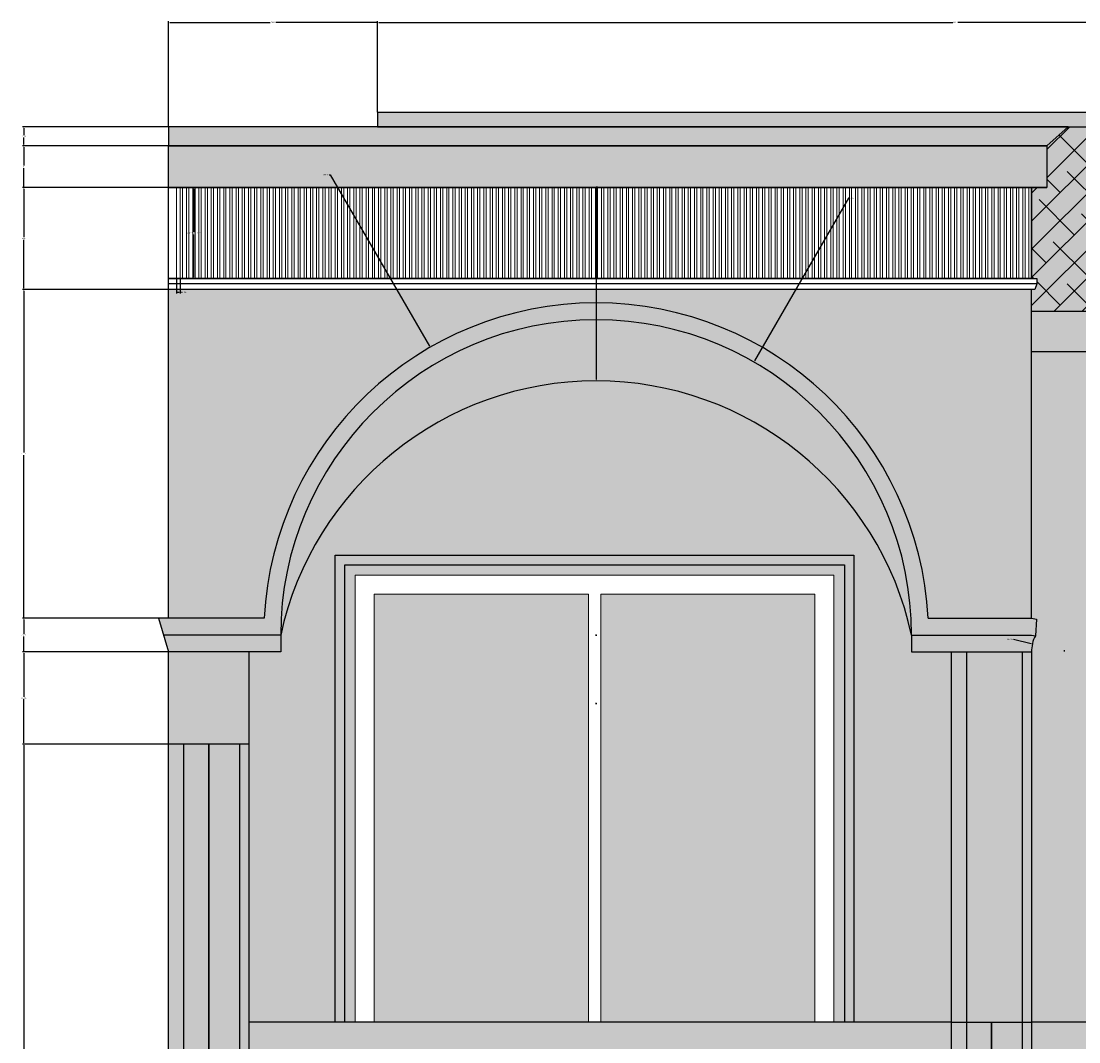
# Model space of a CAD drawing. Units: feet. Extents: x 2352 to 2983, y 950 to 1233.
# Tile 2 of 5: x 2352 to 2504, y 1086 to 1233. Entities that reach past the tile are written whole.
import ezdxf

# ---------------------------------------------------------------- set-up
doc = ezdxf.new("R2010")
doc.units = ezdxf.units.FT
for name, color, linetype, lineweight in [('A-ANNO-DIMS', 2, 'Continuous', 18), ('A-ELEV', 7, 'Continuous', 25), ('A-ELEV-DETL', 8, 'Continuous', 13), ('A-ELEV-PATT', 252, 'Continuous', 13), ('A-GLAZ', 4, 'Continuous', 18)]:
    doc.layers.add(name, color=color, linetype=linetype, lineweight=lineweight)
doc.styles.get("Standard").update_dxf_attribs({"font": 'arial.ttf'})
doc.dimstyles.get("Standard").update_dxf_attribs({"dimtxt": 0.18, "dimasz": 0.18, "dimexe": 0.18, "dimexo": 0.0625, "dimgap": 0.09, "dimtad": 0, "dimtih": 1, "dimtoh": 1, "dimdec": 1, "dimzin": 0, "dimdsep": 46, "dimlunit": 3, "dimtxsty": 'Standard', "dimcen": 0.09, "dimadec": 0, "dimazin": 0, "dimtfac": 1, "dimtdec": 1, "dimtofl": 0, "dimtmove": 0, "dimatfit": 3, "dimfxl": 1, "dimtolj": 1, "dimtzin": 0, "dimarcsym": 0})

# ---------------------------------------------------------------- blocks, each defined once
blk = doc.blocks.new('GRILLE-SLAT')
blk.add_lwpolyline([(0, 13.08), (0.56, 13.08), (0.56, 0), (0, 0)], close=True)
blk.add_lwpolyline([(0, 13.08), (0.56, 13.08), (0.56, 0), (0, 0)], close=True)
blk = doc.blocks.new('*D5')
at = {"layer": 'A-ANNO-DIMS', "color": 0, "lineweight": -2, "transparency": 16777216}
for p, q in [((2375.04, 1209.01), (2377.12, 1209.01)), ((2376.94, 1208.83), (2376.94, 1202.66)), ((2376.94, 1196.12), (2376.94, 1202.29)), ((2375.04, 1195.94), (2377.12, 1195.94))]:
    blk.add_line(p, q, dxfattribs=at)
at = {"layer": 'A-ANNO-DIMS', "color": 0, "transparency": 16777216}
for points in [[(2376.91, 1208.83), (2376.97, 1208.83), (2376.94, 1209.01)], [(2376.91, 1196.12), (2376.97, 1196.12), (2376.94, 1195.94)]]:
    blk.add_solid(points, dxfattribs=at)
at = {"layer": 'Defpoints', "color": 0, "transparency": 16777216}
for p in [(2374.98, 1209.01), (2376.94, 1209.01), (2374.98, 1195.94)]:
    blk.add_point(p, dxfattribs=at)
at = {"layer": 'A-ANNO-DIMS', "color": 0, "transparency": 16777216, "insert": (2376.94, 1202.47), "char_height": 0.18, "attachment_point": 5}
blk.add_mtext('\\A1;GRILLE SLAT 13 TYP.', dxfattribs=at)
blk = doc.blocks.new('*D6')
at = {"layer": 'A-ANNO-DIMS', "color": 0, "lineweight": -2, "transparency": 16777216}
for p, q in [((2374.42, 1195.87), (2374.42, 1193.79)), ((2374.98, 1195.87), (2374.98, 1193.79)), ((2374.6, 1193.97), (2374.8, 1193.97)), ((2374.98, 1193.97), (2375.16, 1193.97))]:
    blk.add_line(p, q, dxfattribs=at)
at = {"layer": 'A-ANNO-DIMS', "color": 0, "transparency": 16777216}
for points in [[(2374.6, 1194), (2374.6, 1193.94), (2374.42, 1193.97)], [(2374.8, 1194), (2374.8, 1193.94), (2374.98, 1193.97)]]:
    blk.add_solid(points, dxfattribs=at)
at = {"layer": 'Defpoints', "color": 0, "transparency": 16777216}
for p in [(2374.42, 1195.94), (2374.98, 1195.94), (2374.98, 1193.97)]:
    blk.add_point(p, dxfattribs=at)
at = {"layer": 'A-ANNO-DIMS', "color": 0, "transparency": 16777216, "insert": (2375.61, 1193.97), "char_height": 0.18, "attachment_point": 5}
blk.add_mtext('\\A1;1 TYP.', dxfattribs=at)
blk = doc.blocks.new('*D8')
at = {"layer": 'A-ANNO-DIMS', "color": 0, "lineweight": -2, "transparency": 16777216}
for p, q in [((2373.3, 1217.81), (2373.3, 1232.95)), ((2403.34, 1219.88), (2403.34, 1232.95)), ((2373.48, 1232.77), (2387.92, 1232.77)), ((2403.16, 1232.77), (2388.71, 1232.77))]:
    blk.add_line(p, q, dxfattribs=at)
at = {"layer": 'A-ANNO-DIMS', "color": 0, "transparency": 16777216}
for points in [[(2373.48, 1232.8), (2373.48, 1232.74), (2373.3, 1232.77)], [(2403.16, 1232.8), (2403.16, 1232.74), (2403.34, 1232.77)]]:
    blk.add_solid(points, dxfattribs=at)
at = {"layer": 'Defpoints', "color": 0, "transparency": 16777216}
for p in [(2403.34, 1232.77), (2403.34, 1219.82), (2373.3, 1217.75)]:
    blk.add_point(p, dxfattribs=at)
at = {"layer": 'A-ANNO-DIMS', "color": 0, "transparency": 16777216, "insert": (2388.32, 1232.77), "char_height": 0.18, "attachment_point": 5}
blk.add_mtext('\\A1;30.04', dxfattribs=at)
blk = doc.blocks.new('*D9')
at = {"layer": 'A-ANNO-DIMS', "color": 0, "lineweight": -2, "transparency": 16777216}
for p, q in [((2403.34, 1219.88), (2403.34, 1232.95)), ((2569.44, 1219.88), (2569.44, 1232.95)), ((2403.52, 1232.77), (2486.02, 1232.77)), ((2569.26, 1232.77), (2486.76, 1232.77))]:
    blk.add_line(p, q, dxfattribs=at)
at = {"layer": 'A-ANNO-DIMS', "color": 0, "transparency": 16777216}
for points in [[(2403.52, 1232.8), (2403.52, 1232.74), (2403.34, 1232.77)], [(2569.26, 1232.8), (2569.26, 1232.74), (2569.44, 1232.77)]]:
    blk.add_solid(points, dxfattribs=at)
at = {"layer": 'Defpoints', "color": 0, "transparency": 16777216}
for p in [(2569.44, 1232.77), (2403.34, 1219.82), (2569.44, 1219.82)]:
    blk.add_point(p, dxfattribs=at)
at = {"layer": 'A-ANNO-DIMS', "color": 0, "transparency": 16777216, "insert": (2486.39, 1232.77), "char_height": 0.18, "attachment_point": 5}
blk.add_mtext('\\A1;166.1', dxfattribs=at)
blk = doc.blocks.new('*D23')
at = {"layer": 'A-ANNO-DIMS', "color": 0, "lineweight": -2, "transparency": 16777216}
for p, q in [((2373.23, 1129.01), (2352.3, 1129.01)), ((2352.48, 1128.83), (2352.48, 1077.3)), ((2352.48, 1025.39), (2352.48, 1076.93)), ((2365.37, 1025.21), (2352.3, 1025.21))]:
    blk.add_line(p, q, dxfattribs=at)
at = {"layer": 'A-ANNO-DIMS', "color": 0, "transparency": 16777216}
for points in [[(2352.45, 1128.83), (2352.51, 1128.83), (2352.48, 1129.01)], [(2352.45, 1025.39), (2352.51, 1025.39), (2352.48, 1025.21)]]:
    blk.add_solid(points, dxfattribs=at)
at = {"layer": 'Defpoints', "color": 0, "transparency": 16777216}
for p in [(2352.48, 1129.01), (2373.3, 1129.01), (2365.43, 1025.21)]:
    blk.add_point(p, dxfattribs=at)
at = {"layer": 'A-ANNO-DIMS', "color": 0, "transparency": 16777216, "insert": (2352.48, 1077.11), "char_height": 0.18, "attachment_point": 5}
blk.add_mtext('\\A1;103.8', dxfattribs=at)
blk = doc.blocks.new('*D24')
at = {"layer": 'A-ANNO-DIMS', "color": 0, "lineweight": -2, "transparency": 16777216}
for p, q in [((2373.23, 1142.24), (2352.3, 1142.24)), ((2352.48, 1142.06), (2352.48, 1135.81)), ((2352.48, 1129.19), (2352.48, 1135.44)), ((2373.23, 1129.01), (2352.3, 1129.01))]:
    blk.add_line(p, q, dxfattribs=at)
at = {"layer": 'A-ANNO-DIMS', "color": 0, "transparency": 16777216}
for points in [[(2352.45, 1142.06), (2352.51, 1142.06), (2352.48, 1142.24)], [(2352.45, 1129.19), (2352.51, 1129.19), (2352.48, 1129.01)]]:
    blk.add_solid(points, dxfattribs=at)
at = {"layer": 'Defpoints', "color": 0, "transparency": 16777216}
for p in [(2352.48, 1142.24), (2373.3, 1142.24), (2373.3, 1129.01)]:
    blk.add_point(p, dxfattribs=at)
at = {"layer": 'A-ANNO-DIMS', "color": 0, "transparency": 16777216, "insert": (2352.48, 1135.63), "char_height": 0.18, "attachment_point": 5}
blk.add_mtext('\\A1;13.224', dxfattribs=at)
blk = doc.blocks.new('*D25')
at = {"layer": 'A-ANNO-DIMS', "color": 0, "lineweight": -2, "transparency": 16777216}
for p, q in [((2371.8, 1147.09), (2352.3, 1147.09)), ((2352.48, 1146.91), (2352.48, 1144.85)), ((2352.48, 1142.42), (2352.48, 1144.48)), ((2373.23, 1142.24), (2352.3, 1142.24))]:
    blk.add_line(p, q, dxfattribs=at)
at = {"layer": 'A-ANNO-DIMS', "color": 0, "transparency": 16777216}
for points in [[(2352.45, 1146.91), (2352.51, 1146.91), (2352.48, 1147.09)], [(2352.45, 1142.42), (2352.51, 1142.42), (2352.48, 1142.24)]]:
    blk.add_solid(points, dxfattribs=at)
at = {"layer": 'Defpoints', "color": 0, "transparency": 16777216}
for p in [(2352.48, 1147.09), (2371.86, 1147.09), (2373.3, 1142.24)]:
    blk.add_point(p, dxfattribs=at)
at = {"layer": 'A-ANNO-DIMS', "color": 0, "transparency": 16777216, "insert": (2352.48, 1144.67), "char_height": 0.18, "attachment_point": 5}
blk.add_mtext('\\A1;4.853', dxfattribs=at)
blk = doc.blocks.new('*D26')
at = {"layer": 'A-ANNO-DIMS', "color": 0, "lineweight": -2, "transparency": 16777216}
for p, q in [((2373.23, 1194.37), (2352.3, 1194.37)), ((2352.48, 1194.19), (2352.48, 1170.91)), ((2352.48, 1147.27), (2352.48, 1170.55)), ((2371.8, 1147.09), (2352.3, 1147.09))]:
    blk.add_line(p, q, dxfattribs=at)
at = {"layer": 'A-ANNO-DIMS', "color": 0, "transparency": 16777216}
for points in [[(2352.45, 1194.19), (2352.51, 1194.19), (2352.48, 1194.37)], [(2352.45, 1147.27), (2352.51, 1147.27), (2352.48, 1147.09)]]:
    blk.add_solid(points, dxfattribs=at)
at = {"layer": 'Defpoints', "color": 0, "transparency": 16777216}
for p in [(2352.48, 1194.37), (2373.3, 1194.37), (2371.86, 1147.09)]:
    blk.add_point(p, dxfattribs=at)
at = {"layer": 'A-ANNO-DIMS', "color": 0, "transparency": 16777216, "insert": (2352.48, 1170.73), "char_height": 0.18, "attachment_point": 5}
blk.add_mtext('\\A1;47.28', dxfattribs=at)
blk = doc.blocks.new('*D27')
at = {"layer": 'A-ANNO-DIMS', "color": 0, "lineweight": -2, "transparency": 16777216}
for p, q in [((2373.23, 1209.01), (2352.3, 1209.01)), ((2352.48, 1208.83), (2352.48, 1201.87)), ((2352.48, 1194.55), (2352.48, 1201.51)), ((2373.23, 1194.37), (2352.3, 1194.37))]:
    blk.add_line(p, q, dxfattribs=at)
at = {"layer": 'A-ANNO-DIMS', "color": 0, "transparency": 16777216}
for points in [[(2352.45, 1208.83), (2352.51, 1208.83), (2352.48, 1209.01)], [(2352.45, 1194.55), (2352.51, 1194.55), (2352.48, 1194.37)]]:
    blk.add_solid(points, dxfattribs=at)
at = {"layer": 'Defpoints', "color": 0, "transparency": 16777216}
for p in [(2352.48, 1209.01), (2373.3, 1209.01), (2373.3, 1194.37)]:
    blk.add_point(p, dxfattribs=at)
at = {"layer": 'A-ANNO-DIMS', "color": 0, "transparency": 16777216, "insert": (2352.48, 1201.69), "char_height": 0.18, "attachment_point": 5}
blk.add_mtext('\\A1;14.64', dxfattribs=at)
blk = doc.blocks.new('*D28')
at = {"layer": 'A-ANNO-DIMS', "color": 0, "lineweight": -2, "transparency": 16777216}
for p, q in [((2373.23, 1215.01), (2352.3, 1215.01)), ((2352.48, 1214.83), (2352.48, 1212.19)), ((2352.48, 1209.19), (2352.48, 1211.83)), ((2373.23, 1209.01), (2352.3, 1209.01))]:
    blk.add_line(p, q, dxfattribs=at)
at = {"layer": 'A-ANNO-DIMS', "color": 0, "transparency": 16777216}
for points in [[(2352.45, 1214.83), (2352.51, 1214.83), (2352.48, 1215.01)], [(2352.45, 1209.19), (2352.51, 1209.19), (2352.48, 1209.01)]]:
    blk.add_solid(points, dxfattribs=at)
at = {"layer": 'Defpoints', "color": 0, "transparency": 16777216}
for p in [(2352.48, 1215.01), (2373.3, 1215.01), (2373.3, 1209.01)]:
    blk.add_point(p, dxfattribs=at)
at = {"layer": 'A-ANNO-DIMS', "color": 0, "transparency": 16777216, "insert": (2352.48, 1212.01), "char_height": 0.18, "attachment_point": 5}
blk.add_mtext('\\A1;6', dxfattribs=at)
blk = doc.blocks.new('*D29')
at = {"layer": 'A-ANNO-DIMS', "color": 0, "lineweight": -2, "transparency": 16777216}
for p, q in [((2373.23, 1217.75), (2352.3, 1217.75)), ((2352.48, 1217.57), (2352.48, 1216.56)), ((2352.48, 1215.19), (2352.48, 1216.2)), ((2373.23, 1215.01), (2352.3, 1215.01))]:
    blk.add_line(p, q, dxfattribs=at)
at = {"layer": 'A-ANNO-DIMS', "color": 0, "transparency": 16777216}
for points in [[(2352.45, 1217.57), (2352.51, 1217.57), (2352.48, 1217.75)], [(2352.45, 1215.19), (2352.51, 1215.19), (2352.48, 1215.01)]]:
    blk.add_solid(points, dxfattribs=at)
at = {"layer": 'Defpoints', "color": 0, "transparency": 16777216}
for p in [(2352.48, 1217.75), (2373.3, 1217.75), (2373.3, 1215.01)]:
    blk.add_point(p, dxfattribs=at)
at = {"layer": 'A-ANNO-DIMS', "color": 0, "transparency": 16777216, "insert": (2352.48, 1216.38), "char_height": 0.18, "attachment_point": 5}
blk.add_mtext('\\A1;2.74', dxfattribs=at)
blk = doc.blocks.new('*D60')
at = {"layer": 'A-ANNO-DIMS', "color": 0, "lineweight": -2, "transparency": 16777216}
for p, q in [((2396.36, 1210.86), (2396.54, 1210.86)), ((2396.54, 1210.86), (2410.78, 1186.19)), ((2434.75, 1144.58), (2434.75, 1144.76)), ((2434.66, 1144.67), (2434.84, 1144.67))]:
    blk.add_line(p, q, dxfattribs=at)
at = {"layer": 'A-ANNO-DIMS', "color": 0, "transparency": 16777216}
blk.add_solid([(2410.8, 1186.21), (2410.75, 1186.18), (2410.87, 1186.03)], dxfattribs=at)
at = {"layer": 'Defpoints', "color": 0, "transparency": 16777216}
for p in [(2410.87, 1186.03), (2434.75, 1144.67)]:
    blk.add_point(p, dxfattribs=at)
at = {"layer": 'A-ANNO-DIMS', "color": 0, "transparency": 16777216, "insert": (2395.88, 1210.86), "char_height": 0.18, "attachment_point": 5}
blk.add_mtext('\\A1;R47.77', dxfattribs=at)
blk = doc.blocks.new('*D61')
at = {"layer": 'A-ANNO-DIMS', "color": 0, "lineweight": -2, "transparency": 16777216}
for p, q in [((2434.93, 1209.06), (2434.75, 1209.06)), ((2434.75, 1209.06), (2434.75, 1181.4)), ((2434.66, 1134.83), (2434.84, 1134.83)), ((2434.75, 1134.74), (2434.75, 1134.92))]:
    blk.add_line(p, q, dxfattribs=at)
at = {"layer": 'A-ANNO-DIMS', "color": 0, "transparency": 16777216}
blk.add_solid([(2434.72, 1181.4), (2434.78, 1181.4), (2434.75, 1181.22)], dxfattribs=at)
at = {"layer": 'Defpoints', "color": 0, "transparency": 16777216}
for p in [(2434.75, 1181.22), (2434.75, 1134.83)]:
    blk.add_point(p, dxfattribs=at)
at = {"layer": 'A-ANNO-DIMS', "color": 0, "transparency": 16777216, "insert": (2435.34, 1209.06), "char_height": 0.18, "attachment_point": 5}
blk.add_mtext('\\A1;R46.4', dxfattribs=at)
blk = doc.blocks.new('*D62')
at = {"layer": 'A-ANNO-DIMS', "color": 0, "lineweight": -2, "transparency": 16777216}
for p, q in [((2471.02, 1207.49), (2457.51, 1184.09)), ((2471.2, 1207.49), (2471.02, 1207.49)), ((2434.75, 1144.58), (2434.75, 1144.76)), ((2434.66, 1144.67), (2434.84, 1144.67))]:
    blk.add_line(p, q, dxfattribs=at)
at = {"layer": 'A-ANNO-DIMS', "color": 0, "transparency": 16777216}
blk.add_solid([(2457.48, 1184.1), (2457.54, 1184.07), (2457.42, 1183.93)], dxfattribs=at)
at = {"layer": 'Defpoints', "color": 0, "transparency": 16777216}
for p in [(2457.42, 1183.93), (2434.75, 1144.67)]:
    blk.add_point(p, dxfattribs=at)
at = {"layer": 'A-ANNO-DIMS', "color": 0, "transparency": 16777216, "insert": (2471.68, 1207.49), "char_height": 0.18, "attachment_point": 5}
blk.add_mtext('\\A1;R45.34', dxfattribs=at)
blk = doc.blocks.new('*D65')
at = {"layer": 'A-ANNO-DIMS', "color": 0, "lineweight": -2, "transparency": 16777216}
for p, q in [((2494.71, 1144.07), (2497.28, 1143.48)), ((2501.95, 1142.41), (2502.13, 1142.41)), ((2502.04, 1142.32), (2502.04, 1142.5))]:
    blk.add_line(p, q, dxfattribs=at)
at = {"layer": 'A-ANNO-DIMS', "color": 0, "transparency": 16777216}
blk.add_solid([(2497.29, 1143.51), (2497.27, 1143.45), (2497.46, 1143.44)], dxfattribs=at)
at = {"layer": 'Defpoints', "color": 0, "transparency": 16777216}
for p in [(2497.46, 1143.44), (2502.04, 1142.41)]:
    blk.add_point(p, dxfattribs=at)
at = {"layer": 'A-ANNO-DIMS', "color": 0, "transparency": 16777216, "insert": (2494.23, 1144.07), "char_height": 0.18, "attachment_point": 5}
blk.add_mtext('\\A1;R4.699', dxfattribs=at)

msp = doc.modelspace()

# ---------------------------------------------------------------- hatches: boundary and pattern name
at = {"layer": 'A-ELEV-PATT'}
h = msp.add_hatch(color=256, dxfattribs=at)
h.dxf.hatch_style = 1
h.paths.add_polyline_path([(2499.5465, 1215.0126), (2373.2965, 1215.0126), (2373.2965, 1209.0126), (2499.5465, 1209.0126)])
h.paths.add_polyline_path([(2502.6085, 1217.7513), (2403.3368, 1217.7513), (2373.2965, 1217.7513), (2373.2965, 1215.0126), (2499.5465, 1215.0126)])
h.paths.add_polyline_path([(2569.4416, 1219.8182), (2403.3368, 1219.8182), (2403.3368, 1217.7513), (2569.4416, 1217.7513)])
h.paths.add_polyline_path([(2593.9663, 1076.1207), (2582.4111, 1069.3398), (2582.4111, 1011.4831), (2595.2079, 1011.4831), (2595.2079, 1023.0126), (2594.1881, 1024.8551), (2594.1881, 1026.3357), (2594.1891, 1026.3338, 0.10932946), (2593.9663, 1027.4578)])
h.paths.add_polyline_path([(2602.5286, 1209.0126), (2593.9663, 1209.0126), (2593.9663, 1027.4578), (2595.2079, 1025.2146), (2602.5286, 1025.2146)])
h.paths.add_polyline_path([(2593.9663, 1083.0126), (2497.3422, 1083.0126), (2497.3422, 1076.1207), (2593.9663, 1076.1207)])
h.paths.add_polyline_path([(2485.8114, 1075.3288), (2384.8273, 1075.3288), (2384.8273, 1011.4831), (2398.2572, 1011.4831), (2398.2572, 1042.4514), (2479.5304, 1042.4514), (2479.5304, 1025.2146), (2485.8114, 1025.2146)])
h.paths.add_polyline_path([(2485.8114, 1083.0126), (2383.4779, 1083.0126), (2383.4779, 1076.1207), (2485.8114, 1076.1207)])
h.paths.add_polyline_path([(2495.9928, 1089.0126), (2491.6239, 1089.0126), (2491.6239, 1025.2146), (2495.9928, 1025.2146)])
h.paths.add_polyline_path([(2491.5297, 1089.0126), (2488.0105, 1089.0126), (2488.0105, 1025.2146), (2491.5297, 1025.2146)])
h.paths.add_polyline_path([(2379.0148, 1129.0147), (2375.4956, 1129.0147), (2375.4956, 1025.2146), (2379.0148, 1025.2146)])
h.paths.add_polyline_path([(2383.4779, 1129.0147), (2379.109, 1129.0147), (2379.109, 1025.2146), (2381.1604, 1025.2146), (2383.4779, 1025.8769)])
h.paths.add_polyline_path([(2389.4076, 1144.6653), (2389.4076, 1142.2389), (2384.8273, 1142.2389), (2384.8273, 1089.0126), (2397.2412, 1089.0126), (2397.2412, 1156.1636), (2471.8066, 1156.1636), (2471.8066, 1089.0126), (2485.8114, 1089.0126), (2485.8114, 1142.2389), (2480.0884, 1142.2389), (2480.0884, 1144.6653, 0.80625477)])
h.paths.add_polyline_path([(2389.4076, 1144.6653, -0.80625477), (2480.0884, 1144.6653, 1)])
h.paths.add_polyline_path([(2579.9743, 1185.4477), (2497.3422, 1185.4477), (2497.3422, 1147.0918), (2498.0576, 1146.9764), (2497.8725, 1144.5798, 0.11184527), (2497.3422, 1142.5724), (2497.3422, 1089.0126), (2505.6415, 1089.0126), (2505.6415, 1159.528, -1), (2532.4859, 1159.528), (2532.4859, 1089.0126), (2541.7346, 1089.0126), (2541.7346, 1159.528, -1), (2568.579, 1159.528), (2568.579, 1089.0126), (2579.9743, 1089.0126)])
h.paths.add_polyline_path([(2579.9743, 1191.2362), (2497.3422, 1191.2362), (2497.3422, 1185.4477), (2579.9743, 1185.4477)])
h.paths.add_polyline_path([(2381.1604, 1023.0126), (2367.0741, 1023.0126), (2367.0741, 963.0126), (2381.1604, 963.0126)])
h.paths.add_polyline_path([(2495.2282, 1011.4831), (2495.2282, 1023.0126), (2439.9479, 1023.0126), (2439.9479, 963.0126), (2446.428, 963.0126), (2446.428, 989.9926, -1), (2485.4222, 989.9926), (2485.4222, 963.0126), (2495.2282, 963.0126)])
h.paths.add_polyline_path([(2446.428, 989.9926), (2446.428, 963.0126), (2485.4222, 963.0126), (2485.4222, 989.9926, 1)], flags=17)
h.paths.add_polyline_path([(2603.7702, 1023.0126), (2595.2079, 1023.0126), (2595.2079, 1011.4831), (2595.2079, 963.0126), (2603.7702, 963.0126)])
h.paths.add_polyline_path([(2482.4531, 1147.0918), (2497.3422, 1147.0918), (2497.3422, 1185.4477), (2497.3422, 1194.3715), (2373.2965, 1194.3715), (2373.2965, 1147.0918), (2387.0428, 1147.0918, -0.95042953)])
h.paths.add_polyline_path([(2384.8273, 1142.2389), (2373.2965, 1142.2389), (2373.2965, 1129.0147), (2384.8273, 1129.0147)])
h.paths.add_polyline_path([(2495.9928, 1142.2389), (2488.0105, 1142.2389), (2488.0105, 1089.0126), (2491.5297, 1089.0126), (2495.9928, 1089.0126)])
h = msp.add_hatch(color=256, dxfattribs=at)
h.dxf.hatch_style = 1
h.paths.add_polyline_path([(2595.2079, 1011.4831), (2495.2282, 1011.4831), (2495.2282, 963.0126), (2595.2079, 963.0126)])
h.paths.add_polyline_path([(2579.9743, 1204.1231), (2569.4416, 1217.7513), (2502.6085, 1217.7513), (2499.5465, 1215.0126), (2499.5465, 1209.0126), (2497.3422, 1209.0126), (2497.3422, 1195.936), (2498.0772, 1195.936), (2498.0772, 1195.1775), (2497.8022, 1194.3715), (2497.3422, 1194.3715), (2497.3422, 1191.2362), (2579.9743, 1191.2362)])
h = msp.add_hatch(dxfattribs=at)
h.set_pattern_fill('ANSI38', color=256, scale=0.9)
h.paths.add_polyline_path([(2569.4416, 1217.7513), (2502.6085, 1217.7513), (2499.5465, 1215.0126), (2499.5465, 1209.0126), (2497.3422, 1209.0126), (2497.3422, 1195.936), (2498.0772, 1195.936), (2498.0772, 1195.1775), (2497.8022, 1194.3715), (2497.3422, 1194.3715), (2497.3422, 1191.2362), (2579.9743, 1191.2362), (2579.9743, 1204.1231)])
h.paths.add_polyline_path([(2579.9743, 1204.1231), (2579.9743, 1191.2362), (2589.9732, 1191.1856)])
h = msp.add_hatch(color=256, dxfattribs=at)
h.dxf.hatch_style = 1
h.paths.add_polyline_path([(2480.0884, 1144.6653), (2497.3422, 1144.6653), (2497.8725, 1144.5798), (2498.0576, 1146.9764), (2497.3422, 1147.0918), (2482.4531, 1147.0918, 0.95042953), (2387.0428, 1147.0918), (2373.2965, 1147.0918), (2371.8622, 1147.0918), (2372.5793, 1144.6653), (2389.4076, 1144.6653, -1)])
h.paths.add_polyline_path([(2389.4076, 1144.6653), (2372.5793, 1144.6653), (2373.2965, 1142.2389), (2389.4076, 1142.2389)])
h.paths.add_polyline_path([(2497.8725, 1144.5798), (2497.3422, 1144.6653), (2480.0884, 1144.6653), (2480.0884, 1142.2389), (2497.3422, 1142.2389, -0.12985075)])
h.paths.add_polyline_path([(2471.8066, 1156.1636), (2397.2412, 1156.1636), (2397.2412, 1089.0126), (2398.6146, 1089.0126), (2398.6146, 1154.7902), (2470.4332, 1154.7902), (2470.4332, 1089.0126), (2471.8066, 1089.0126)])
h.paths.add_polyline_path([(2470.4332, 1154.7902), (2398.6146, 1154.7902), (2398.6146, 1089.0126), (2400.114, 1089.0126), (2400.114, 1153.2908), (2468.9338, 1153.2908), (2468.9338, 1089.0126), (2470.4332, 1089.0126)], flags=17)
h.paths.add_polyline_path([(2495.8508, 1024.4932), (2439.2183, 1024.4932), (2439.2183, 1023.0126), (2495.8508, 1023.0126)])
h.paths.add_polyline_path([(2496.3417, 1025.2146), (2438.7275, 1025.2146, -0.22451739), (2439.2183, 1024.4932), (2495.8508, 1024.4932, -0.22451739)])
h.paths.add_polyline_path([(2381.1604, 1024.4932), (2366.1676, 1024.4932), (2366.1676, 1023.0126), (2381.1604, 1023.0126)])
h.paths.add_polyline_path([(2381.1604, 1025.2146), (2365.4325, 1025.2146, -0.12196493), (2366.1676, 1024.4932), (2381.1604, 1024.4932)])
h.paths.add_polyline_path([(2383.4779, 1025.1555), (2383.4779, 1025.8769), (2381.1604, 1025.2146), (2381.1604, 1024.4932)])
h.paths.add_polyline_path([(2383.4779, 1025.1555), (2381.1604, 1024.4932), (2381.1604, 1023.0126), (2383.4779, 1023.6749)])
h.paths.add_polyline_path([(2479.5304, 1042.4514), (2398.2572, 1042.4514), (2398.2572, 1011.4831), (2399.3703, 1011.4831), (2399.3703, 1041.3383), (2478.4174, 1041.3383), (2478.4174, 1025.2146), (2479.5304, 1025.2146)])
h.paths.add_polyline_path([(2478.4174, 1041.3383), (2399.3703, 1041.3383), (2399.3703, 1011.4831), (2400.6982, 1011.4831), (2400.6982, 1040.0104), (2477.0895, 1040.0104), (2477.0895, 1025.2146), (2478.4174, 1025.2146)], flags=17)
h.paths.add_polyline_path([(2565.0085, 1048.4289), (2535.3542, 1048.4289), (2535.3542, 1011.4831), (2536.3698, 1011.4831), (2536.3698, 1047.4133), (2563.993, 1047.4133), (2563.993, 1011.4831), (2565.0085, 1011.4831)])
h.paths.add_polyline_path([(2522.2926, 1048.4289), (2497.3422, 1048.4289), (2497.3422, 1047.4929), (2521.3566, 1047.4929), (2521.3566, 1011.4831), (2522.2926, 1011.4831)])
h.paths.add_polyline_path([(2603.9449, 1025.2146), (2603.7702, 1025.2146), (2595.2079, 1025.2146), (2593.9663, 1027.4578, -0.10932946), (2594.1891, 1026.3338), (2595.2079, 1024.4932), (2603.7702, 1024.4932, -0.10758073)])
h.paths.add_polyline_path([(2603.7702, 1024.4932), (2595.2079, 1024.4932), (2594.1891, 1026.3338, -0.00342101), (2594.1881, 1026.2975), (2594.1881, 1024.8551), (2595.2079, 1023.0126), (2603.7702, 1023.0126)])
h.paths.add_polyline_path([(2532.4859, 1159.528, 1), (2505.6415, 1159.528), (2505.6415, 1089.0126), (2505.9696, 1089.0126), (2505.9696, 1126.273), (2505.9696, 1159.528, -1), (2532.1578, 1159.528), (2532.1578, 1089.0126), (2532.4859, 1089.0126)])
h.paths.add_polyline_path([(2542.0627, 1159.528, -1), (2568.2509, 1159.528), (2568.2509, 1089.0126), (2568.579, 1089.0126), (2568.579, 1159.528, 1), (2541.7346, 1159.528), (2541.7346, 1089.0126), (2542.0627, 1089.0126)])
h.paths.add_polyline_path([(2522.687, 1127.7792), (2505.9696, 1127.7792), (2505.9696, 1126.273), (2511.9257, 1126.273), (2511.9257, 1089.0126), (2512.1488, 1089.0126), (2512.1488, 1126.273), (2521.1808, 1126.273), (2521.1808, 1089.0126), (2522.687, 1089.0126)], flags=17)
h.paths.add_polyline_path([(2439.9479, 1011.4831), (2381.1604, 1011.4831), (2381.1604, 963.0126), (2439.9479, 963.0126)])
h = msp.add_hatch(color=256, dxfattribs=at)
h.dxf.hatch_style = 1
h.paths.add_polyline_path([(2438.1858, 1039.4184), (2401.2902, 1039.4184), (2401.2902, 1011.4831), (2438.1858, 1011.4831)])
h.paths.add_polyline_path([(2476.4975, 1039.4184), (2440.2408, 1039.4184), (2440.2408, 1025.2146), (2476.4975, 1025.2146)])
h.paths.add_polyline_path([(2563.252, 1046.6724), (2550.43, 1046.6724), (2550.43, 1011.4831), (2563.252, 1011.4831)])
h.paths.add_polyline_path([(2549.9328, 1046.6724), (2537.1107, 1046.6724), (2537.1107, 1011.4831), (2549.9328, 1011.4831)])
h.paths.add_polyline_path([(2520.4416, 1046.5779), (2507.7848, 1046.5779), (2507.7848, 1011.4831), (2520.4416, 1011.4831)])
h.paths.add_polyline_path([(2506.8593, 1046.5779), (2497.3422, 1046.5779), (2497.3422, 1011.4831), (2506.8593, 1011.4831)])
h.paths.add_polyline_path([(2521.1808, 1126.273), (2512.1488, 1126.273), (2512.1488, 1089.0126), (2521.1808, 1089.0126)])
h.paths.add_polyline_path([(2511.9257, 1126.273), (2505.9696, 1126.273), (2505.9696, 1089.0126), (2511.9257, 1089.0126)])
h.paths.add_polyline_path([(2466.1883, 1150.5453), (2435.4142, 1150.5453), (2435.4142, 1089.0126), (2466.1883, 1089.0126)])
h.paths.add_polyline_path([(2433.6336, 1150.5453), (2402.8595, 1150.5453), (2402.8595, 1089.0126), (2433.6336, 1089.0126)])
h = msp.add_hatch(color=256, dxfattribs=at)
h.dxf.hatch_style = 1
h.paths.add_polyline_path([(2593.9663, 1089.0126), (2497.3422, 1089.0126), (2497.3422, 1083.0126), (2593.9663, 1083.0126)])
h.paths.add_polyline_path([(2485.8114, 1089.0126), (2384.8273, 1089.0126), (2384.8273, 1083.0126), (2485.8114, 1083.0126)])
h.paths.add_polyline_path([(2375.4956, 1129.0147), (2373.2965, 1129.0147), (2373.2965, 1025.2146), (2375.4956, 1025.2146)])
h.paths.add_polyline_path([(2384.8273, 1129.0147), (2383.4779, 1129.0147), (2383.4779, 1083.0126), (2384.8273, 1083.0126)])
h.paths.add_polyline_path([(2384.8273, 1075.3288), (2383.4779, 1076.1207), (2383.4779, 1025.8769), (2383.4779, 1011.4831), (2384.8273, 1011.4831)])
h.paths.add_polyline_path([(2488.0105, 1089.0126), (2485.8114, 1089.0126), (2485.8114, 1025.2146), (2488.0105, 1025.2146)])
h.paths.add_polyline_path([(2497.3422, 1089.0126), (2495.9928, 1089.0126), (2495.9928, 1025.2146), (2496.3417, 1025.2146, 0.22451739), (2495.8508, 1024.4932), (2495.8508, 1023.0126), (2495.2282, 1023.0126), (2495.2282, 1011.4831), (2497.3422, 1011.4831), (2497.3422, 1048.4289)])
h.paths.add_polyline_path([(2497.3422, 1142.2389), (2495.9928, 1142.2389), (2495.9928, 1089.0126), (2497.3422, 1089.0126)])
h.paths.add_polyline_path([(2488.0105, 1142.2389), (2485.8114, 1142.2389), (2485.8114, 1089.0126), (2488.0105, 1089.0126)])

# ---------------------------------------------------------------- linework, layer by layer
at = {"layer": 'A-ELEV'}
for p, q in [((2499.5465, 1215.0126), (2502.6085, 1217.7513)), ((2499.5465, 1215.0126), (2502.6085, 1217.7513)), ((2499.5465, 1215.0126), (2373.2965, 1215.0126)), ((2499.5465, 1215.0126), (2373.2965, 1215.0126)), ((2373.2965, 1209.0126), (2499.5465, 1209.0126)), ((2373.2965, 1209.0126), (2499.5465, 1209.0126)), ((2497.3422, 1195.936), (2497.3422, 1209.0126)), ((2497.3422, 1195.936), (2497.3422, 1209.0126)), ((2498.0772, 1195.1775), (2497.8022, 1194.3715)), ((2498.0772, 1195.1775), (2497.8022, 1194.3715)), ((2497.3422, 1194.3715), (2373.2965, 1194.3715)), ((2497.3422, 1194.3715), (2373.2965, 1194.3715)), ((2497.8022, 1194.3715), (2497.3422, 1194.3715)), ((2497.3422, 1147.0918), (2497.3422, 1194.3715)), ((2497.8022, 1194.3715), (2497.3422, 1194.3715)), ((2497.3422, 1191.2362), (2579.9743, 1191.2362)), ((2497.3422, 1191.2362), (2589.9341, 1191.2362)), ((2497.3422, 1185.4477), (2593.9663, 1185.4477)), ((2373.2965, 1147.0918), (2371.8622, 1147.0918)), ((2371.8622, 1147.0918), (2373.2965, 1142.2389)), ((2373.2965, 1147.0918), (2371.8622, 1147.0918)), ((2371.8622, 1147.0918), (2373.2965, 1142.2389)), ((2387.0428, 1147.0918), (2373.2965, 1147.0918)), ((2387.0428, 1147.0918), (2373.2965, 1147.0918)), ((2482.4531, 1147.0918), (2497.3422, 1147.0918)), ((2482.4531, 1147.0918), (2497.3422, 1147.0918)), ((2497.3422, 1147.0918), (2498.0576, 1146.9764)), ((2497.3422, 1147.0918), (2498.0576, 1146.9764)), ((2498.0576, 1146.9764), (2497.8725, 1144.5798)), ((2498.0576, 1146.9764), (2497.8725, 1144.5798)), ((2389.4076, 1144.6653), (2372.5793, 1144.6653)), ((2389.4076, 1144.6653), (2372.5793, 1144.6653)), ((2389.4076, 1144.6653), (2389.4076, 1142.2389)), ((2389.4076, 1144.6653), (2389.4076, 1142.2389)), ((2480.0884, 1144.6653), (2497.3422, 1144.6653)), ((2480.0884, 1144.6653), (2480.0884, 1142.2389)), ((2480.0884, 1144.6653), (2497.3422, 1144.6653)), ((2480.0884, 1144.6653), (2480.0884, 1142.2389)), ((2497.3422, 1144.6653), (2497.8725, 1144.5798)), ((2497.3422, 1144.6653), (2497.8725, 1144.5798)), ((2389.4076, 1142.2389), (2373.2965, 1142.2389)), ((2389.4076, 1142.2389), (2373.2965, 1142.2389)), ((2480.0884, 1142.2389), (2497.3422, 1142.2389)), ((2480.0884, 1142.2389), (2497.3422, 1142.2389)), ((2373.2965, 1129.0147), (2384.8273, 1129.0147)), ((2373.2965, 1129.0147), (2384.8273, 1129.0147)), ((2485.8114, 1089.0126), (2384.8273, 1089.0126)), ((2485.8114, 1089.0126), (2384.8273, 1089.0126)), ((2485.8114, 1089.0126), (2497.3422, 1089.0126)), ((2485.8114, 1089.0126), (2497.3422, 1089.0126)), ((2593.9663, 1089.0126), (2497.3422, 1089.0126)), ((2593.9663, 1089.0126), (2497.3422, 1089.0126))]:
    msp.add_line(p, q, dxfattribs=at)
for points in [[(2403.3368, 1217.7513), (2569.4416, 1217.7513), (2569.4416, 1219.8182), (2403.3368, 1219.8182)], [(2403.3368, 1217.7513), (2569.4416, 1217.7513), (2569.4416, 1219.8182), (2403.3368, 1219.8182)], [(2373.2965, 1215.0126), (2499.5465, 1215.0126), (2499.5465, 1209.0126), (2373.2965, 1209.0126)], [(2373.2965, 1215.0126), (2499.5465, 1215.0126), (2499.5465, 1209.0126), (2373.2965, 1209.0126)], [(2373.2965, 1209.0126), (2497.3422, 1209.0126), (2497.3422, 1195.936), (2373.2965, 1195.936)], [(2373.2965, 1209.0126), (2497.3422, 1209.0126), (2497.3422, 1195.936), (2373.2965, 1195.936)], [(2498.0772, 1195.1775), (2373.2965, 1195.1775), (2373.2965, 1195.936), (2498.0772, 1195.936)], [(2498.0772, 1195.1775), (2373.2965, 1195.1775), (2373.2965, 1195.936), (2498.0772, 1195.936)], [(2471.8066, 1089.0126), (2397.2412, 1089.0126), (2397.2412, 1156.1636), (2471.8066, 1156.1636)], [(2471.8066, 1089.0126), (2397.2412, 1089.0126), (2397.2412, 1156.1636), (2471.8066, 1156.1636)]]:
    msp.add_lwpolyline(points, close=True, dxfattribs=at)
for points in [[(2502.6085, 1217.7513), (2373.2965, 1217.7513), (2373.2965, 1215.0126), (2499.5465, 1215.0126)], [(2502.6085, 1217.7513), (2373.2965, 1217.7513), (2373.2965, 1215.0126), (2499.5465, 1215.0126)], [(2373.2965, 1147.0918), (2373.2965, 1215.0126)], [(2373.2965, 1147.0918), (2373.2965, 1215.0126)], [(2491.6239, 1215.0126), (2491.5297, 1215.0126)], [(2491.6239, 1215.0126), (2491.5297, 1215.0126)], [(2398.6146, 1089.0126), (2398.6146, 1154.7902), (2470.4332, 1154.7902), (2470.4332, 1089.0126)], [(2398.6146, 1089.0126), (2398.6146, 1154.7902), (2470.4332, 1154.7902), (2470.4332, 1089.0126)], [(2373.2965, 1025.2146), (2373.2965, 1142.2389)], [(2373.2965, 1025.2146), (2373.2965, 1142.2389)], [(2384.8273, 1142.2389), (2384.8273, 1083.0126)], [(2384.8273, 1142.2389), (2384.8273, 1083.0126)], [(2485.8114, 1025.2146), (2485.8114, 1142.2389)], [(2485.8114, 1025.2146), (2485.8114, 1142.2389)], [(2488.0105, 1025.2146), (2488.0105, 1142.2389)], [(2488.0105, 1025.2146), (2488.0105, 1142.2389)], [(2495.9928, 1142.2389), (2495.9928, 1025.2146)], [(2495.9928, 1142.2389), (2495.9928, 1025.2146)], [(2497.3422, 1142.5724), (2497.3422, 1011.4831)], [(2497.3422, 1142.5724), (2497.3422, 1011.4831)], [(2375.4956, 1025.2146), (2375.4956, 1129.0147)], [(2375.4956, 1025.2146), (2375.4956, 1129.0147)], [(2379.0148, 1129.0147), (2379.0148, 1025.2146), (2379.109, 1025.2146), (2379.109, 1129.0147)], [(2379.0148, 1129.0147), (2379.0148, 1025.2146), (2379.109, 1025.2146), (2379.109, 1129.0147)], [(2383.4779, 1129.0147), (2383.4779, 1025.8769)], [(2383.4779, 1129.0147), (2383.4779, 1025.8769)], [(2491.5297, 1089.0126), (2491.5297, 1025.2146), (2491.6239, 1025.2146), (2491.6239, 1089.0126)], [(2491.5297, 1089.0126), (2491.5297, 1025.2146), (2491.6239, 1025.2146), (2491.6239, 1089.0126)]]:
    msp.add_lwpolyline(points, dxfattribs=at)
for centre, radius, start, end in [((2434.748, 1144.6653), 47.7668, 2.911736, 177.088264), ((2434.748, 1144.6653), 47.7668, 2.911736, 177.088264), ((2434.748, 1144.6653), 45.3404, 0, 180), ((2434.748, 1144.6653), 45.3404, 0, 180), ((2434.748, 1134.8254), 46.3959, 12.244676, 167.755324), ((2434.748, 1134.8254), 46.3959, 12.244676, 167.755324), ((2502.0383, 1142.4056), 4.699, 152.439516, 182.033526), ((2502.0383, 1142.4056), 4.699, 152.439516, 182.033526)]:
    msp.add_arc(centre, radius, start, end, dxfattribs=at)
at = {"layer": 'A-GLAZ'}
for points in [[(2400.114, 1089.0126), (2400.114, 1153.2908), (2468.9338, 1153.2908), (2468.9338, 1089.0126)], [(2400.114, 1089.0126), (2400.114, 1153.2908), (2468.9338, 1153.2908), (2468.9338, 1089.0126)], [(2402.8595, 1089.0126), (2402.8595, 1150.5453), (2433.6336, 1150.5453)], [(2402.8595, 1089.0126), (2402.8595, 1150.5453), (2433.6336, 1150.5453)], [(2435.4142, 1150.5453), (2435.4142, 1089.0126), (2433.6336, 1089.0126), (2433.6336, 1150.5453)], [(2435.4142, 1150.5453), (2435.4142, 1089.0126), (2433.6336, 1089.0126), (2433.6336, 1150.5453)], [(2435.4142, 1150.5453), (2466.1883, 1150.5453), (2466.1883, 1089.0126)], [(2435.4142, 1150.5453), (2466.1883, 1150.5453), (2466.1883, 1089.0126)]]:
    msp.add_lwpolyline(points, dxfattribs=at)

# ---------------------------------------------------------------- block references
at = {"layer": 'A-ELEV-DETL'}
for p in [(2374.424, 1195.936), (2375.3143, 1195.936), (2376.2047, 1195.936), (2377.095, 1195.936), (2377.9853, 1195.936), (2378.8757, 1195.936), (2379.766, 1195.936), (2380.6563, 1195.936), (2381.5467, 1195.936), (2382.437, 1195.936), (2383.3273, 1195.936), (2384.2177, 1195.936), (2385.108, 1195.936), (2385.9983, 1195.936), (2386.8887, 1195.936), (2387.779, 1195.936), (2388.6693, 1195.936), (2389.5597, 1195.936), (2390.45, 1195.936), (2391.3403, 1195.936), (2392.2307, 1195.936), (2393.121, 1195.936), (2394.0113, 1195.936), (2394.9017, 1195.936), (2395.792, 1195.936), (2396.6823, 1195.936), (2397.5727, 1195.936), (2398.463, 1195.936), (2399.3533, 1195.936), (2400.2436, 1195.936), (2401.134, 1195.936), (2402.0243, 1195.936), (2402.9146, 1195.936), (2403.805, 1195.936), (2404.6953, 1195.936), (2405.5856, 1195.936), (2406.476, 1195.936), (2407.3663, 1195.936), (2408.2566, 1195.936), (2409.147, 1195.936), (2410.0373, 1195.936), (2410.9276, 1195.936), (2411.818, 1195.936), (2412.7083, 1195.936), (2413.5986, 1195.936), (2414.489, 1195.936), (2415.3793, 1195.936), (2416.2696, 1195.936), (2417.16, 1195.936), (2418.0503, 1195.936), (2418.9406, 1195.936), (2419.831, 1195.936), (2420.7213, 1195.936), (2421.6116, 1195.936), (2422.502, 1195.936), (2423.3923, 1195.936), (2424.2826, 1195.936), (2425.173, 1195.936), (2426.0633, 1195.936), (2426.9536, 1195.936), (2427.844, 1195.936), (2428.7343, 1195.936), (2429.6246, 1195.936), (2430.515, 1195.936), (2431.4053, 1195.936), (2432.2956, 1195.936), (2433.186, 1195.936), (2434.0763, 1195.936), (2434.9666, 1195.936), (2435.857, 1195.936), (2436.7473, 1195.936), (2437.6376, 1195.936), (2438.528, 1195.936), (2439.4183, 1195.936), (2440.3086, 1195.936), (2441.199, 1195.936), (2442.0893, 1195.936), (2442.9796, 1195.936), (2443.87, 1195.936), (2444.7603, 1195.936), (2445.6506, 1195.936), (2446.541, 1195.936), (2447.4313, 1195.936), (2448.3216, 1195.936), (2449.2119, 1195.936), (2450.1023, 1195.936), (2450.9926, 1195.936), (2451.8829, 1195.936), (2452.7733, 1195.936), (2453.6636, 1195.936), (2454.5539, 1195.936), (2455.4443, 1195.936), (2456.3346, 1195.936), (2457.2249, 1195.936), (2458.1153, 1195.936), (2459.0056, 1195.936), (2459.8959, 1195.936), (2460.7863, 1195.936), (2461.6766, 1195.936), (2462.5669, 1195.936), (2463.4573, 1195.936), (2464.3476, 1195.936), (2465.2379, 1195.936), (2466.1283, 1195.936), (2467.0186, 1195.936), (2467.9089, 1195.936), (2468.7993, 1195.936), (2469.6896, 1195.936), (2470.5799, 1195.936), (2471.4703, 1195.936), (2472.3606, 1195.936), (2473.2509, 1195.936), (2474.1413, 1195.936), (2475.0316, 1195.936), (2475.9219, 1195.936), (2476.8123, 1195.936), (2477.7026, 1195.936), (2478.5929, 1195.936), (2479.4833, 1195.936), (2480.3736, 1195.936), (2481.2639, 1195.936), (2482.1543, 1195.936), (2483.0446, 1195.936), (2483.9349, 1195.936), (2484.8253, 1195.936), (2485.7156, 1195.936), (2486.6059, 1195.936), (2487.4963, 1195.936), (2488.3866, 1195.936), (2489.2769, 1195.936), (2490.1673, 1195.936), (2491.0576, 1195.936), (2491.9479, 1195.936), (2492.8383, 1195.936), (2493.7286, 1195.936), (2494.6189, 1195.936), (2495.5093, 1195.936), (2496.3996, 1195.936)]:
    msp.add_blockref('GRILLE-SLAT', p, dxfattribs=at)

# ---------------------------------------------------------------- dimensions: what is measured, and where the dimension line sits
at = {"layer": 'A-ANNO-DIMS'}
for base, p1, p2, override, picture, middle in [((2403.3368, 1232.7682), (2373.2965, 1217.7513), (2403.3368, 1219.8182), {"dimdec": 2, "dimlfac": 1, "dimrnd": 0, "dimzin": 0, "dimdsep": 46, "dimlunit": 2}, '*D8', (2388.3167, 1232.7682)), ((2569.4416, 1232.7682), (2403.3368, 1219.8182), (2569.4416, 1219.8182), {"dimdec": 1, "dimlfac": 1, "dimrnd": 0, "dimzin": 0, "dimdsep": 46, "dimlunit": 2}, '*D9', (2486.3892, 1232.7682))]:
    dim = msp.add_linear_dim(base=base, p1=p1, p2=p2, dimstyle='Standard', override=override, dxfattribs=at)
    dim.commit()
    dim.dimension.update_dxf_attribs({"geometry": picture, "text_midpoint": middle})
for base, p1, p2, override, picture, middle in [((2352.4825, 1217.7513), (2373.2965, 1215.0126), (2373.2965, 1217.7513), {"dimdec": 2, "dimlfac": 1, "dimrnd": 0, "dimzin": 0, "dimdsep": 46, "dimlunit": 2}, '*D29', (2352.4825, 1216.382)), ((2352.4825, 1215.0126), (2373.2965, 1209.0126), (2373.2965, 1215.0126), {"dimdec": 0, "dimlfac": 1, "dimrnd": 0, "dimzin": 0, "dimdsep": 46, "dimlunit": 2}, '*D28', (2352.4825, 1212.0126)), ((2352.4825, 1209.0126), (2373.2965, 1194.3715), (2373.2965, 1209.0126), {"dimdec": 2, "dimlfac": 1, "dimrnd": 0, "dimzin": 0, "dimdsep": 46, "dimlunit": 2}, '*D27', (2352.4825, 1201.6921)), ((2352.4825, 1194.3715), (2371.8622, 1147.0918), (2373.2965, 1194.3715), {"dimdec": 2, "dimlfac": 1, "dimrnd": 0, "dimzin": 0, "dimdsep": 46, "dimlunit": 2}, '*D26', (2352.4825, 1170.7317)), ((2352.4825, 1147.0918), (2373.2965, 1142.2389), (2371.8622, 1147.0918), {"dimdec": 3, "dimlfac": 1, "dimrnd": 0, "dimzin": 0, "dimdsep": 46, "dimlunit": 2}, '*D25', (2352.4825, 1144.6653)), ((2352.4825, 1142.2389), (2373.2965, 1129.0147), (2373.2965, 1142.2389), {"dimdec": 3, "dimlfac": 1, "dimrnd": 0, "dimzin": 0, "dimdsep": 46, "dimlunit": 2}, '*D24', (2352.4825, 1135.6268)), ((2352.4825, 1129.0147), (2365.4325, 1025.2146), (2373.2965, 1129.0147), {"dimdec": 1, "dimlfac": 1, "dimrnd": 0, "dimzin": 0, "dimdsep": 46, "dimlunit": 2}, '*D23', (2352.4825, 1077.1147))]:
    dim = msp.add_linear_dim(base=base, p1=p1, p2=p2, angle=90, dimstyle='Standard', override=override, dxfattribs=at)
    dim.commit()
    dim.dimension.update_dxf_attribs({"geometry": picture, "text_midpoint": middle})
for center, mpoint, override, picture, middle in [((2434.748, 1144.6653), (2410.8675, 1186.0343), {"dimdec": 2, "dimlfac": 1, "dimrnd": 0, "dimzin": 0, "dimdsep": 46, "dimlunit": 2}, '*D60', (2395.8794, 1210.8557)), ((2434.748, 1134.8254), (2434.748, 1181.2212), {"dimdec": 1, "dimlfac": 1, "dimrnd": 0, "dimzin": 0, "dimdsep": 46, "dimlunit": 2}, '*D61', (2435.3375, 1209.0587)), ((2434.748, 1144.6653), (2457.4201, 1183.9302), {"dimdec": 2, "dimlfac": 1, "dimrnd": 0, "dimzin": 0, "dimdsep": 46, "dimlunit": 2}, '*D62', (2471.6828, 1207.489)), ((2502.0383, 1142.4056), (2497.4554, 1143.4439), {"dimdec": 3, "dimlfac": 1, "dimrnd": 0, "dimzin": 0, "dimdsep": 46, "dimlunit": 2}, '*D65', (2494.7057, 1144.0669))]:
    dim = msp.add_radius_dim(center=center, mpoint=mpoint, dimstyle='Standard', override=override, dxfattribs=at)
    dim.commit()
    dim.dimension.update_dxf_attribs({"geometry": picture, "text_midpoint": middle, "dimtype": 164})
dim = msp.add_linear_dim(base=(2376.943, 1209.0126), p1=(2374.9816, 1195.936), p2=(2374.9816, 1209.0126), angle=90, text='GRILLE SLAT <> TYP.', dimstyle='Standard', override={"dimdec": 0, "dimrnd": 0, "dimzin": 0, "dimlunit": 2}, dxfattribs=at)
dim.commit()
dim.dimension.update_dxf_attribs({"geometry": '*D5', "text_midpoint": (2376.943, 1202.4743)})
dim = msp.add_linear_dim(base=(2374.9816, 1193.9745), p1=(2374.4239, 1195.936), p2=(2374.9816, 1195.936), text='<> TYP.', dimstyle='Standard', override={"dimdec": 0, "dimrnd": 0, "dimzin": 0, "dimlunit": 2}, dxfattribs=at)
dim.commit()
dim.dimension.update_dxf_attribs({"geometry": '*D6', "text_midpoint": (2375.6112, 1193.9745)})

doc.saveas('drawing.dxf')
